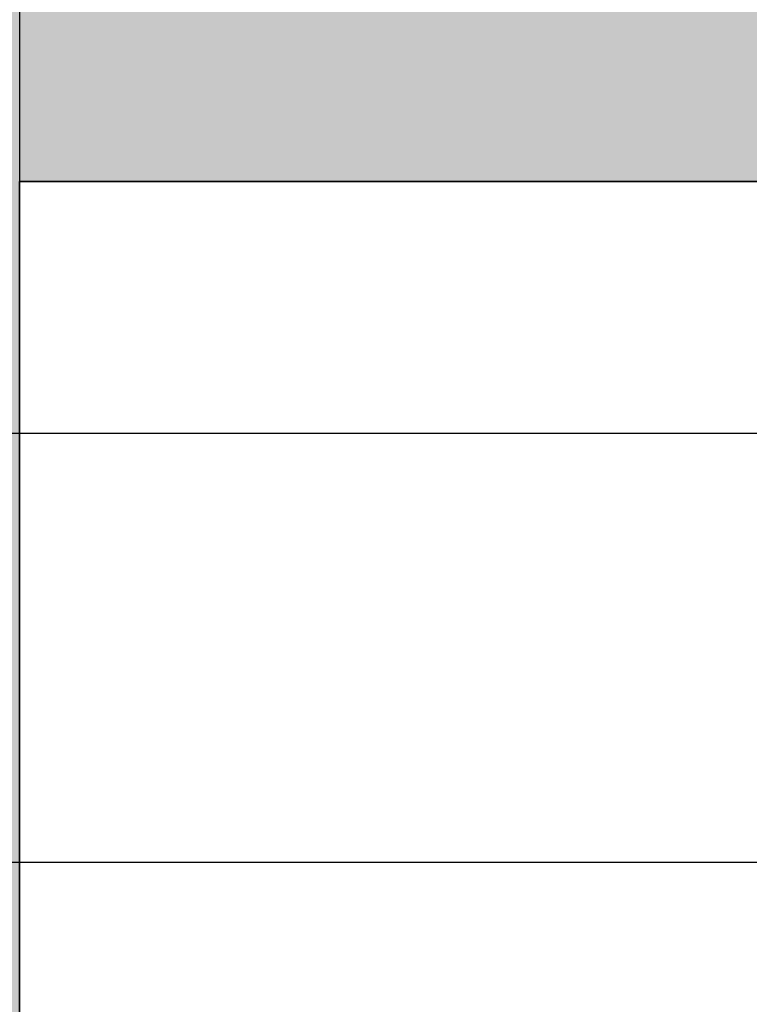
# Model space of a CAD drawing. Units: inches. Extents: x 2696 to 3240, y 1564 to 2310.
# Tile 16 of 76: x 2755 to 2769, y 1890 to 1910. Entities that reach past the tile are written whole.
import ezdxf

# ---------------------------------------------------------------- set-up
doc = ezdxf.new("R2010")
doc.units = ezdxf.units.IN
for name, color, linetype, lineweight in [('A-ANNO-DIMS', 3, 'Continuous', 18), ('A-WALL', 7, 'Continuous', 35), ('A-WALL-PATT', 9, 'Continuous', 13)]:
    doc.layers.add(name, color=color, linetype=linetype, lineweight=lineweight)
doc.styles.add('TIMES NEW', font='times.ttf')
doc.dimstyles.new('Siddhuu', dxfattribs={"dimtxt": 6, "dimasz": 2.5, "dimexe": 1.25, "dimexo": 0.625, "dimtad": 1, "dimdec": 1, "dimlunit": 4, "dimtxsty": 'TIMES NEW', "dimcen": 2.5, "dimclrd": 256, "dimclre": 1, "dimclrt": 7, "dimadec": 0, "dimazin": 0, "dimtfac": 1, "dimtdec": 1, "dimtmove": 0, "dimatfit": 3, "dimfxl": 1, "dimtolj": 1, "dimlwd": -1, "dimarcsym": 0})

# ---------------------------------------------------------------- blocks, each defined once
blk = doc.blocks.new('*D55')
at = {"layer": 'A-ANNO-DIMS', "color": 1, "lineweight": -2, "transparency": 16777216}
for p, q in [((3189.986, 1980.201), (2709.361, 1980.201)), ((3189.986, 1893.201), (2709.361, 1893.201))]:
    blk.add_line(p, q, dxfattribs=at)
at = {"layer": 'A-ANNO-DIMS', "transparency": 16777216}
blk.add_line((2710.611, 1895.701), (2710.611, 1977.701), dxfattribs=at)
for points in [[(2710.195, 1977.701), (2711.028, 1977.701), (2710.611, 1980.201)], [(2710.195, 1895.701), (2711.028, 1895.701), (2710.611, 1893.201)]]:
    blk.add_solid(points, dxfattribs=at)
at = {"layer": 'Defpoints', "color": 0, "transparency": 16777216}
for p in [(2710.611, 1980.201), (3190.611, 1980.201), (3190.611, 1893.201)]:
    blk.add_point(p, dxfattribs=at)
at = {"layer": 'A-ANNO-DIMS', "color": 7, "transparency": 16777216, "insert": (2706.926, 1936.701), "char_height": 6, "attachment_point": 5, "rotation": 90, "style": 'TIMES NEW'}
blk.add_mtext('\\A1;7\'-3"', dxfattribs=at)
blk = doc.blocks.new('*D57')
at = {"layer": 'A-ANNO-DIMS', "color": 1, "lineweight": -2, "transparency": 16777216}
for p, q in [((2754.611, 2018.576), (2754.611, 1568.951)), ((2956.709, 2018.576), (2956.709, 1568.951))]:
    blk.add_line(p, q, dxfattribs=at)
at = {"layer": 'A-ANNO-DIMS', "transparency": 16777216}
blk.add_line((2757.111, 1570.201), (2954.209, 1570.201), dxfattribs=at)
for points in [[(2757.111, 1570.618), (2757.111, 1569.784), (2754.611, 1570.201)], [(2954.209, 1570.618), (2954.209, 1569.784), (2956.709, 1570.201)]]:
    blk.add_solid(points, dxfattribs=at)
at = {"layer": 'Defpoints', "color": 0, "transparency": 16777216}
for p in [(2754.611, 2019.201), (2956.709, 2019.201), (2956.709, 1570.201)]:
    blk.add_point(p, dxfattribs=at)
at = {"layer": 'A-ANNO-DIMS', "color": 7, "transparency": 16777216, "insert": (2855.66, 1573.878), "char_height": 6, "attachment_point": 5, "style": 'TIMES NEW'}
blk.add_mtext('\\A1;16\'-10"', dxfattribs=at)
blk = doc.blocks.new('*D68')
at = {"layer": 'A-ANNO-DIMS', "color": 1, "lineweight": -2, "transparency": 16777216}
for p, q in [((2745.611, 2261.576), (2745.611, 1568.951)), ((2782.834, 2261.576), (2782.834, 1568.951))]:
    blk.add_line(p, q, dxfattribs=at)
at = {"layer": 'A-ANNO-DIMS', "transparency": 16777216}
blk.add_line((2748.111, 1570.201), (2780.334, 1570.201), dxfattribs=at)
for points in [[(2748.111, 1570.618), (2748.111, 1569.784), (2745.611, 1570.201)], [(2780.334, 1570.618), (2780.334, 1569.784), (2782.834, 1570.201)]]:
    blk.add_solid(points, dxfattribs=at)
at = {"layer": 'Defpoints', "color": 0, "transparency": 16777216}
for p in [(2745.611, 2262.201), (2782.834, 2262.201), (2782.834, 1570.201)]:
    blk.add_point(p, dxfattribs=at)
at = {"layer": 'A-ANNO-DIMS', "color": 7, "transparency": 16777216, "insert": (2764.223, 1573.878), "char_height": 6, "attachment_point": 5, "style": 'TIMES NEW'}
blk.add_mtext('\\A1;3\'-1"', dxfattribs=at)
blk = doc.blocks.new('*D78')
at = {"layer": 'A-ANNO-DIMS', "transparency": 16777216}
for p, q in [((2710.611, 1901.701), (2710.611, 1935.101)), ((2710.611, 1895.701), (2710.611, 1899.201))]:
    blk.add_line(p, q, dxfattribs=at)
at = {"layer": 'A-ANNO-DIMS', "color": 1, "lineweight": -2, "transparency": 16777216}
for p, q in [((3189.986, 1901.701), (2709.361, 1901.701)), ((3189.986, 1893.201), (2709.361, 1893.201))]:
    blk.add_line(p, q, dxfattribs=at)
at = {"layer": 'A-ANNO-DIMS', "transparency": 16777216}
for points in [[(2710.195, 1899.201), (2711.028, 1899.201), (2710.611, 1901.701)], [(2710.195, 1895.701), (2711.028, 1895.701), (2710.611, 1893.201)]]:
    blk.add_solid(points, dxfattribs=at)
at = {"layer": 'Defpoints', "color": 0, "transparency": 16777216}
for p in [(2710.611, 1901.701), (3190.611, 1901.701), (3190.611, 1893.201)]:
    blk.add_point(p, dxfattribs=at)
at = {"layer": 'A-ANNO-DIMS', "color": 7, "transparency": 16777216, "insert": (2706.85, 1919.651), "char_height": 6, "attachment_point": 5, "rotation": 90, "style": 'TIMES NEW'}
blk.add_mtext('\\A1;0\'-8 1/2"', dxfattribs=at)

msp = doc.modelspace()

# ---------------------------------------------------------------- hatches: boundary and pattern name
at = {"layer": 'A-WALL-PATT', "transparency": 33554556}
h = msp.add_hatch(color=256, dxfattribs=at)
h.dxf.hatch_style = 1
h.paths.add_polyline_path([(2879.111, 2253.201), (2905.91, 2253.201), (2905.91, 2262.201), (2841.889, 2262.201), (2841.889, 2253.201), (2870.111, 2253.201), (2870.111, 2176.601), (2965.709, 2176.601), (2965.709, 2206.701), (2973.583, 2206.701), (2973.583, 2215.701), (2965.709, 2215.701), (2965.709, 2262.201), (2929.91, 2262.201), (2929.91, 2253.201), (2956.709, 2253.201), (2956.709, 2185.601), (2879.111, 2185.601)])
h.paths.add_polyline_path([(2782.834, 2262.201), (2745.611, 2262.201), (2745.611, 2228.729), (2754.611, 2228.729), (2754.611, 2253.201), (2782.834, 2253.201)])
h.paths.add_polyline_path([(2754.611, 2136.201), (2965.709, 2136.201), (2965.709, 2145.201), (2879.111, 2145.201), (2879.111, 2147.074), (2877.34, 2147.074), (2870.111, 2147.074), (2870.111, 2145.201), (2754.611, 2145.201), (2754.611, 2169.674), (2745.611, 2169.674), (2745.611, 2000.201), (2754.611, 2000.201), (2754.611, 2019.201), (2849.083, 2019.201), (2849.083, 2023.701), (2841.209, 2023.701), (2841.209, 2051.827), (2836.709, 2051.827), (2836.709, 2023.701), (2754.611, 2023.701), (2754.611, 2091.201), (2836.709, 2091.201), (2836.709, 2087.827), (2841.209, 2087.827), (2841.209, 2095.701), (2754.611, 2095.701)])
h.paths.add_polyline_path([(2965.709, 2136.201), (2956.709, 2136.201), (2956.709, 2023.701), (2885.083, 2023.701), (2885.083, 2019.201), (2956.709, 2019.201), (2956.709, 1950.575), (2965.709, 1950.575), (2965.709, 1980.201), (2973.583, 1980.201), (2973.583, 1989.201), (2965.709, 1989.201)])
h.paths.add_polyline_path([(2754.611, 1906.701), (2880.209, 1906.701), (2884.709, 1906.701), (2956.709, 1906.701), (2956.709, 1792.701), (2944.709, 1792.701), (2944.709, 1783.701), (2956.709, 1783.701), (2956.709, 1740.201), (2884.709, 1740.201), (2884.709, 1783.701), (2896.709, 1783.701), (2896.709, 1792.701), (2884.709, 1792.701), (2884.709, 1846.701), (2880.209, 1846.701), (2880.209, 1740.201), (2754.611, 1740.201), (2754.611, 1777.201), (2745.611, 1777.201), (2745.611, 1692.701), (2754.611, 1692.701), (2754.611, 1731.201), (2956.709, 1731.201), (2956.709, 1723.327), (2965.709, 1723.327), (2965.709, 1884.201), (2973.583, 1884.201), (2973.583, 1893.201), (2965.709, 1893.201), (2965.709, 1914.575), (2956.709, 1914.575), (2956.709, 1911.201), (2754.611, 1911.201), (2754.611, 1930.201), (2745.611, 1930.201), (2745.611, 1817.201), (2754.611, 1817.201), (2754.611, 1854.201), (2826.611, 1854.201), (2826.611, 1868.827), (2822.111, 1868.827), (2822.111, 1858.701), (2754.611, 1858.701)])
h.paths.add_polyline_path([(2965.709, 1656.201), (3008.237, 1656.201), (3008.237, 1665.201), (2965.709, 1665.201), (2965.709, 1693.327), (2956.709, 1693.327), (2956.709, 1686.201), (2934.583, 1686.201), (2934.583, 1681.701), (2956.709, 1681.701), (2956.709, 1614.201), (2896.709, 1614.201), (2896.709, 1681.701), (2904.583, 1681.701), (2904.583, 1686.201), (2892.209, 1686.201), (2892.209, 1614.201), (2858.41, 1614.201), (2858.41, 1605.201), (2965.709, 1605.201)])
h.paths.add_polyline_path([(2788.41, 1614.201), (2754.611, 1614.201), (2754.611, 1652.701), (2745.611, 1652.701), (2745.611, 1605.201), (2788.41, 1605.201)])
h.paths.add_polyline_path([(3199.611, 1633.048), (3190.611, 1633.048), (3190.611, 1614.201), (3082.611, 1614.201), (3082.611, 1665.201), (3070.237, 1665.201), (3070.237, 1656.201), (3078.111, 1656.201), (3078.111, 1605.201), (3199.611, 1605.201)])
h.paths.add_polyline_path([(3199.611, 1702.048), (3190.611, 1702.048), (3190.611, 1699.701), (3106.611, 1699.701), (3106.611, 1747.701), (3190.611, 1747.701), (3190.611, 1752.201), (3082.611, 1752.201), (3082.611, 1760.075), (3078.111, 1760.075), (3078.111, 1747.701), (3102.111, 1747.701), (3102.111, 1699.701), (3078.111, 1699.701), (3078.111, 1695.201), (3190.611, 1695.201), (3190.611, 1676.355), (3199.611, 1676.355)])
h.paths.add_polyline_path([(3199.611, 1783.201), (3190.611, 1783.201), (3190.611, 1745.355), (3199.611, 1745.355)])
h.paths.add_polyline_path([(3082.611, 1884.201), (3190.611, 1884.201), (3190.611, 1853.201), (3199.611, 1853.201), (3199.611, 1901.701), (3190.611, 1901.701), (3190.611, 1893.201), (3005.583, 1893.201), (3005.583, 1891.281), (3005.583, 1884.201), (3078.111, 1884.201), (3078.111, 1792.075), (3082.611, 1792.075)])
h.paths.add_polyline_path([(3199.611, 1994.701), (3190.611, 1994.701), (3190.611, 1989.201), (3073.709, 1989.201), (3073.709, 2034.201), (3069.209, 2034.201), (3069.209, 1989.201), (3005.583, 1989.201), (3005.583, 1980.201), (3190.611, 1980.201), (3190.611, 1971.701), (3199.611, 1971.701)])
h.paths.add_polyline_path([(3199.611, 2155.201), (3190.611, 2155.201), (3190.611, 2064.701), (3199.611, 2064.701)])
h.paths.add_polyline_path([(3190.611, 2074.701), (3106.611, 2074.701), (3106.611, 2122.701), (3190.611, 2122.701), (3190.611, 2127.201), (3082.709, 2127.201), (3082.709, 2135.075), (3073.709, 2135.075), (3073.709, 2122.701), (3102.111, 2122.701), (3102.111, 2074.701), (3069.209, 2074.701), (3069.209, 2070.201), (3190.611, 2070.201)])
h.paths.add_polyline_path([(3082.709, 2253.201), (3190.611, 2253.201), (3190.611, 2225.201), (3199.611, 2225.201), (3199.611, 2262.201), (3073.709, 2262.201), (3073.709, 2215.701), (3035.583, 2215.701), (3035.583, 2206.701), (3073.709, 2206.701), (3073.709, 2171.075), (3082.709, 2171.075)])

# ---------------------------------------------------------------- linework, layer by layer
at = {"layer": 'A-WALL'}
for p, q in [((2754.611, 1906.701), (2880.209, 1906.701)), ((2754.611, 1858.701), (2754.611, 1906.701))]:
    msp.add_line(p, q, dxfattribs=at)

# ---------------------------------------------------------------- dimensions: what is measured, and where the dimension line sits
at = {"layer": 'A-ANNO-DIMS'}
for base, p1, p2, picture, middle in [((2782.834, 1570.201), (2745.611, 2262.201), (2782.834, 2262.201), '*D68', (2764.223, 1573.878)), ((2956.709, 1570.201), (2754.611, 2019.201), (2956.709, 2019.201), '*D57', (2855.66, 1573.878))]:
    dim = msp.add_linear_dim(base=base, p1=p1, p2=p2, dimstyle='Siddhuu', override={"dimdec": 1, "dimlfac": 1, "dimrnd": 0, "dimzin": 1, "dimdsep": 46, "dimlunit": 4, "dimfrac": 2}, dxfattribs=at)
    dim.commit()
    dim.dimension.update_dxf_attribs({"geometry": picture, "text_midpoint": middle})
for base, p2, picture, middle in [((2710.611, 1980.201), (3190.611, 1980.201), '*D55', (2706.926, 1936.701)), ((2710.611, 1901.701), (3190.611, 1901.701), '*D78', (2706.85, 1919.651))]:
    dim = msp.add_linear_dim(base=base, p1=(3190.611, 1893.201), p2=p2, angle=90, dimstyle='Siddhuu', override={"dimdec": 1, "dimlfac": 1, "dimrnd": 0, "dimzin": 1, "dimdsep": 46, "dimlunit": 4, "dimfrac": 2}, dxfattribs=at)
    dim.commit()
    dim.dimension.update_dxf_attribs({"geometry": picture, "text_midpoint": middle})

doc.saveas('drawing.dxf')
